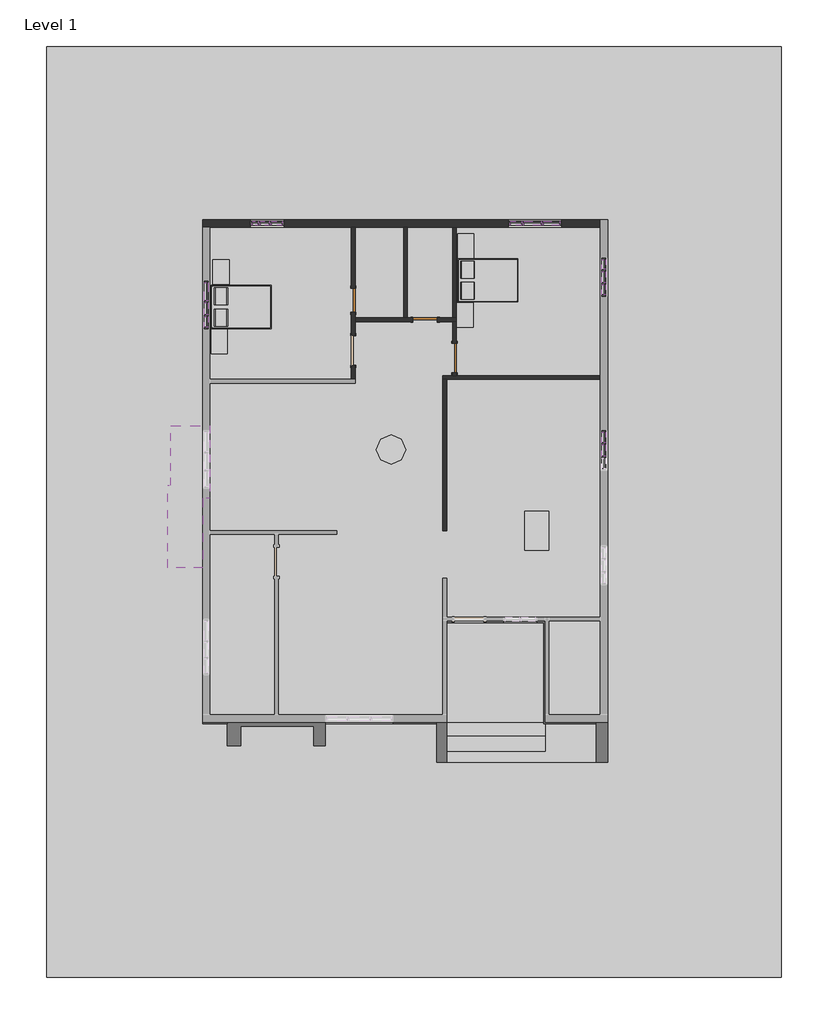
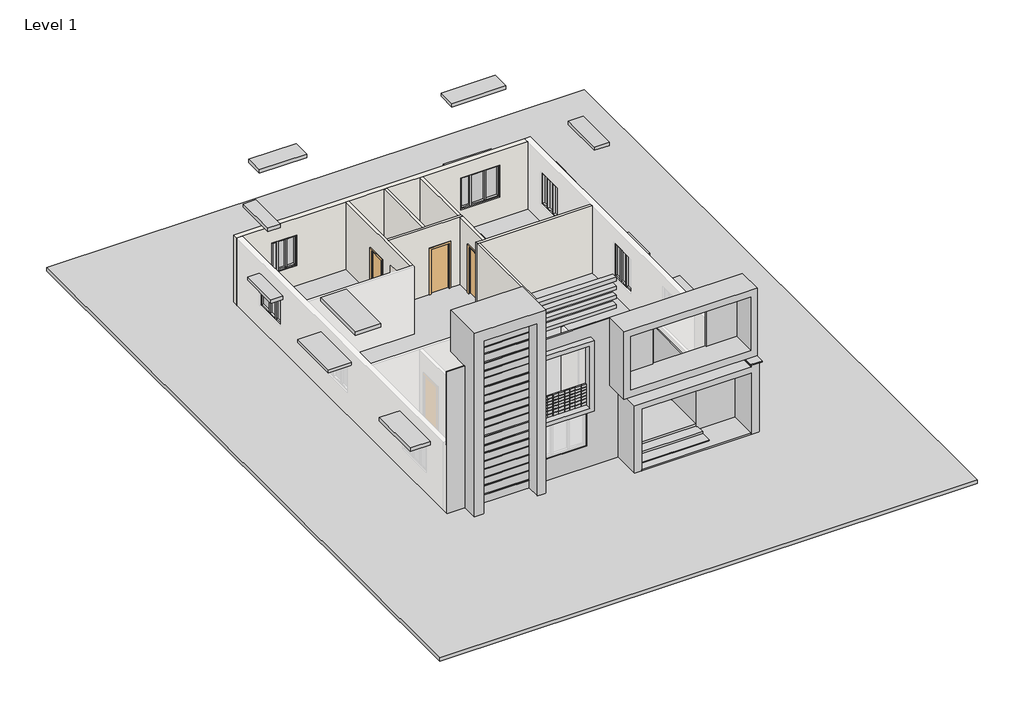
# One storey, part 2 of 2: 48 members, 14 plates, 8 furniture elements, 8 walls, 5 proxies, 3 doors.
"""IFC4 building model written with IfcOpenShell, lengths in millimetres."""

from ifc_helpers import new_model, si_unit, frame, origin, origin_with_axes, place, context, project, spatial, polyline, outline, extrude, faceted_brep, transform, mapped, element, save
from components import generic_models_1_generic_models_1_92a5afb8, generic_models_2_generic_models_2_c2d7a446, generic_models_3_generic_models_3_41235341, generic_models_4_generic_models_4_67bf9aa9, generic_models_6_generic_models_6_d9953a67, door_d8f5dbb5, door_f2b275c1, door_e5f9f3c4, furniture_b58f7881, furniture_fb07e05e, furniture_acc2807d, furniture_52f35bf4, member_ff1b7d8f, member_5ad95953, member_843225dc, member_ff9f2d30, member_49b269a4, member_6edf370a, member_39e99675, member_b57d713a, member_a980948f, member_0b7646a3, member_25243d18, member_408948b5, member_177aa30a, member_02b8d6b6, member_f68f0f88, member_d76d04ed, member_9890e23f, member_83c59054, member_6f432376, member_640288a7, member_b98e8178, system_panel_glazed_4b443884, system_panel_glazed_03b7eec7, system_panel_glazed_fe9977b0, system_panel_glazed_4bf0fdf0, system_panel_glazed_6a6571f5, system_panel_glazed_c4277b2e, system_panel_glazed_5760ca47, system_panel_glazed_ce423334, system_panel_glazed_199a1f6c, system_panel_glazed_e70e5af4, system_panel_glazed_65e788ca, system_panel_glazed_f9e68b79, system_panel_glazed_f010d5cf

model = new_model("IFC4")

# Units and contexts
model_context = context("Model", 3, world=origin())
ifc_project = project(units=[si_unit("LENGTHUNIT", "METRE", prefix="MILLI")], contexts=[model_context])

# Site, building, storey
site = spatial("IfcSite", under=ifc_project)
building = spatial("IfcBuilding", under=site)
storey = spatial("IfcBuildingStorey", under=building, Name="Level 1", Elevation=0.0)

# Proxies
placement = place(None, origin())
generic_models_1_generic_models_1_shape = generic_models_1_generic_models_1_92a5afb8(model_context)
element("IfcBuildingElementProxy", 1, Name="Generic Models 1 : Generic Models 1", ObjectType="Generic Models 1 : Generic Models 1", at=placement, inside=storey, context=model_context, shape_type="MappedRepresentation", body=[
    mapped(generic_models_1_generic_models_1_shape, transform((0.0, 0.0, 0.0), x_axis=(1.0, 0.0, 0.0), y_axis=(0.0, 1.0, 0.0), z_axis=(0.0, 0.0, 1.0))),
])
generic_models_2_generic_models_2_shape = generic_models_2_generic_models_2_c2d7a446(model_context)
element("IfcBuildingElementProxy", 2, Name="Generic Models 2 : Generic Models 2", ObjectType="Generic Models 2 : Generic Models 2", at=placement, inside=storey, context=model_context, shape_type="MappedRepresentation", body=[
    mapped(generic_models_2_generic_models_2_shape, transform((0.0, 0.0, 0.0), x_axis=(1.0, 0.0, 0.0), y_axis=(0.0, 1.0, 0.0), z_axis=(0.0, 0.0, 1.0))),
])
generic_models_3_generic_models_3_shape = generic_models_3_generic_models_3_41235341(model_context)
element("IfcBuildingElementProxy", 3, Name="Generic Models 3 : Generic Models 3", ObjectType="Generic Models 3 : Generic Models 3", at=placement, inside=storey, context=model_context, shape_type="MappedRepresentation", body=[
    mapped(generic_models_3_generic_models_3_shape, transform((0.0, 0.0, 0.0), x_axis=(1.0, 0.0, 0.0), y_axis=(0.0, 1.0, 0.0), z_axis=(0.0, 0.0, 1.0))),
])
generic_models_4_generic_models_4_shape = generic_models_4_generic_models_4_67bf9aa9(model_context)
element("IfcBuildingElementProxy", 4, Name="Generic Models 4 : Generic Models 4", ObjectType="Generic Models 4 : Generic Models 4", at=placement, inside=storey, context=model_context, shape_type="MappedRepresentation", body=[
    mapped(generic_models_4_generic_models_4_shape, transform((0.0, 0.0, 0.0), x_axis=(1.0, 0.0, 0.0), y_axis=(0.0, 1.0, 0.0), z_axis=(0.0, 0.0, 1.0))),
])
generic_models_6_generic_models_6_shape = generic_models_6_generic_models_6_d9953a67(model_context)
element("IfcBuildingElementProxy", 5, Name="Generic Models 6 : Generic Models 6", ObjectType="Generic Models 6 : Generic Models 6", at=placement, inside=storey, context=model_context, shape_type="MappedRepresentation", body=[
    mapped(generic_models_6_generic_models_6_shape, transform((0.0, 0.0, 0.0), x_axis=(1.0, 0.0, 0.0), y_axis=(0.0, 1.0, 0.0), z_axis=(0.0, 0.0, 1.0))),
])

# Doors
door_shape = door_d8f5dbb5(model_context)
element("IfcDoor", 6, ObjectType="Single-Flush : 30\" x 80\"", at=placement, inside=storey, context=model_context, shape_type="MappedRepresentation", body=[
    mapped(door_shape, transform((-18760.1886697, 977.9488046, 0.0), x_axis=(0.0, -1.0, 0.0), y_axis=(1.0, 0.0, 0.0), z_axis=(0.0, 0.0, 1.0))),
])
door_2_shape = door_f2b275c1(model_context)
element("IfcDoor", 7, ObjectType="Single-Flush : 30\" x 80\"", at=placement, inside=storey, context=model_context, shape_type="MappedRepresentation", body=[
    mapped(door_2_shape, transform((-16512.2886697, 368.3488046, 0.0), x_axis=(-1.0, 0.0, 0.0), y_axis=(0.0, -1.0, 0.0), z_axis=(0.0, 0.0, 1.0))),
])
door_3_shape = door_e5f9f3c4(model_context)
element("IfcDoor", 8, ObjectType="Single-Flush : 36\" x 84\"", at=placement, inside=storey, context=model_context, shape_type="MappedRepresentation", body=[
    mapped(door_3_shape, transform((-15597.8886697, -831.8011954, 0.0), x_axis=(0.0, -1.0, 0.0), y_axis=(1.0, 0.0, 0.0), z_axis=(0.0, 0.0, 1.0))),
])

# Furniture
furniture_shape = furniture_b58f7881(model_context)
element("IfcFurniture", 9, ObjectType="Bed-Box : Double 53\" x 74\"", at=placement, inside=storey, context=model_context, shape_type="MappedRepresentation", body=[
    mapped(furniture_shape, transform((-22493.4681779, 425.4988046, 0.0), x_axis=(0.0, 1.0, 0.0), y_axis=(-1.0, 0.0, 0.0), z_axis=(0.0, 0.0, 1.0))),
])
element("IfcFurniture", 10, ObjectType="Bed-Box : Double 53\" x 74\"", at=placement, inside=storey, context=model_context, shape_type="MappedRepresentation", body=[
    mapped(furniture_shape, transform((-14790.9181779, 1261.0963456, 0.0), x_axis=(0.0, 1.0, 0.0), y_axis=(-1.0, 0.0, 0.0), z_axis=(0.0, 0.0, 1.0))),
])
furniture_2_shape = furniture_fb07e05e(model_context)
element("IfcFurniture", 11, ObjectType="Cabinet File-Lateral 3 Drawer : 30\" x 20\" x 36\"", at=placement, inside=storey, context=model_context, shape_type="MappedRepresentation", body=[
    mapped(furniture_2_shape, transform((-23828.3570458, 2034.2713186, 0.0), x_axis=(0.0, 1.0, 0.0), y_axis=(-1.0, 0.0, 0.0), z_axis=(0.0, 0.0, 1.0))),
])
element("IfcFurniture", 12, ObjectType="Cabinet File-Lateral 3 Drawer : 30\" x 20\" x 36\"", at=placement, inside=storey, context=model_context, shape_type="MappedRepresentation", body=[
    mapped(furniture_2_shape, transform((-23879.1570458, -137.4286814, 0.0), x_axis=(0.0, 1.0, 0.0), y_axis=(-1.0, 0.0, 0.0), z_axis=(0.0, 0.0, 1.0))),
])
element("IfcFurniture", 13, ObjectType="Cabinet File-Lateral 3 Drawer : 30\" x 20\" x 36\"", at=placement, inside=storey, context=model_context, shape_type="MappedRepresentation", body=[
    mapped(furniture_2_shape, transform((-16176.6070458, 2847.0713186, 0.0), x_axis=(0.0, 1.0, 0.0), y_axis=(-1.0, 0.0, 0.0), z_axis=(0.0, 0.0, 1.0))),
])
element("IfcFurniture", 14, ObjectType="Cabinet File-Lateral 3 Drawer : 30\" x 20\" x 36\"", at=placement, inside=storey, context=model_context, shape_type="MappedRepresentation", body=[
    mapped(furniture_2_shape, transform((-16202.0070458, 700.7713186, 0.0), x_axis=(0.0, 1.0, 0.0), y_axis=(-1.0, 0.0, 0.0), z_axis=(0.0, 0.0, 1.0))),
])
furniture_3_shape = furniture_acc2807d(model_context)
element("IfcFurniture", 15, ObjectType="Table-Coffee Rectangular : 48\" x 30\"", at=placement, inside=storey, context=model_context, shape_type="MappedRepresentation", body=[
    mapped(furniture_3_shape, transform((-12656.5278379, -6836.2848256, 0.0), x_axis=(0.0, 1.0, 0.0), y_axis=(-1.0, 0.0, 0.0), z_axis=(0.0, 0.0, 1.0))),
])
furniture_4_shape = furniture_52f35bf4(model_context)
element("IfcFurniture", 16, ObjectType="Table-Dining Round w Chairs : 36\" Diameter", at=placement, inside=storey, context=model_context, shape_type="MappedRepresentation", body=[
    mapped(furniture_4_shape, transform((-17682.7706369, -3504.4225068, 0.0), x_axis=(1.0, 0.0, 0.0), y_axis=(0.0, 1.0, 0.0), z_axis=(0.0, 0.0, 1.0))),
])

# Members
member_shape = member_ff1b7d8f(model_context)
element("IfcMember", 17, ObjectType="Rectangular Mullion : 2.5\" x 5\" rectangular", at=placement, inside=storey, context=model_context, shape_type="MappedRepresentation", body=[
    mapped(member_shape, transform((-10930.6386697, 1530.3988046, 2267.0732017), x_axis=(0.0, 0.0, 1.0), y_axis=(-1.0, 0.0, 0.0), z_axis=(0.0, -1.0, 0.0))),
])
member_2_shape = member_5ad95953(model_context)
element("IfcMember", 18, ObjectType="Rectangular Mullion : 2.5\" x 5\" rectangular", at=placement, inside=storey, context=model_context, shape_type="MappedRepresentation", body=[
    mapped(member_2_shape, transform((-10930.6386697, 1936.7988046, 2267.0732017), x_axis=(0.0, 0.0, 1.0), y_axis=(-1.0, 0.0, 0.0), z_axis=(0.0, -1.0, 0.0))),
])
element("IfcMember", 19, ObjectType="Rectangular Mullion : 2.5\" x 5\" rectangular", at=placement, inside=storey, context=model_context, shape_type="MappedRepresentation", body=[
    mapped(member_2_shape, transform((-10930.6386697, 1155.7488046, 2267.0732017), x_axis=(0.0, 0.0, 1.0), y_axis=(-1.0, 0.0, 0.0), z_axis=(0.0, -1.0, 0.0))),
])
element("IfcMember", 20, ObjectType="Rectangular Mullion : 2.5\" x 5\" rectangular", at=placement, inside=storey, context=model_context, shape_type="MappedRepresentation", body=[
    mapped(member_2_shape, transform((-10930.6386697, 1466.8988046, 809.8934331), x_axis=(0.0, 0.0, -1.0), y_axis=(-1.0, 0.0, 0.0), z_axis=(0.0, 1.0, 0.0))),
])
element("IfcMember", 21, ObjectType="Rectangular Mullion : 2.5\" x 5\" rectangular", at=placement, inside=storey, context=model_context, shape_type="MappedRepresentation", body=[
    mapped(member_2_shape, transform((-10930.6386697, 2247.9488046, 809.8934331), x_axis=(0.0, 0.0, -1.0), y_axis=(-1.0, 0.0, 0.0), z_axis=(0.0, 1.0, 0.0))),
])
element("IfcMember", 22, ObjectType="Rectangular Mullion : 2.5\" x 5\" rectangular", at=placement, inside=storey, context=model_context, shape_type="MappedRepresentation", body=[
    mapped(member_shape, transform((-10930.6386697, 1873.2988046, 809.8934331), x_axis=(0.0, 0.0, -1.0), y_axis=(-1.0, 0.0, 0.0), z_axis=(0.0, 1.0, 0.0))),
])
member_3_shape = member_843225dc(model_context)
element("IfcMember", 23, ObjectType="Rectangular Mullion : 2.5\" x 5\" rectangular", at=placement, inside=storey, context=model_context, shape_type="MappedRepresentation", body=[
    mapped(member_3_shape, transform((-10930.6386697, -3536.9011954, 821.4712655), x_axis=(0.0, 0.0, -1.0), y_axis=(-1.0, 0.0, 0.0), z_axis=(0.0, 1.0, 0.0))),
])
element("IfcMember", 24, ObjectType="Rectangular Mullion : 2.5\" x 5\" rectangular", at=placement, inside=storey, context=model_context, shape_type="MappedRepresentation", body=[
    mapped(member_3_shape, transform((-13857.9886697, 3378.2488046, 969.97905), x_axis=(0.0, 0.0, -1.0), y_axis=(0.0, -1.0, 0.0), z_axis=(-1.0, 0.0, 0.0))),
])
member_4_shape = member_ff9f2d30(model_context)
element("IfcMember", 25, ObjectType="Rectangular Mullion : 2.5\" x 5\" rectangular", at=placement, inside=storey, context=model_context, shape_type="MappedRepresentation", body=[
    mapped(member_4_shape, transform((-10930.6386697, -3962.3511954, 821.4712655), x_axis=(0.0, 0.0, -1.0), y_axis=(-1.0, 0.0, 0.0), z_axis=(0.0, 1.0, 0.0))),
])
element("IfcMember", 26, ObjectType="Rectangular Mullion : 2.5\" x 5\" rectangular", at=placement, inside=storey, context=model_context, shape_type="MappedRepresentation", body=[
    mapped(member_4_shape, transform((-10930.6386697, -3143.2011954, 821.4712655), x_axis=(0.0, 0.0, -1.0), y_axis=(-1.0, 0.0, 0.0), z_axis=(0.0, 1.0, 0.0))),
])
member_5_shape = member_49b269a4(model_context)
element("IfcMember", 27, ObjectType="Rectangular Mullion : 2.5\" x 5\" rectangular", at=placement, inside=storey, context=model_context, shape_type="MappedRepresentation", body=[
    mapped(member_5_shape, transform((-10930.6386697, -3930.6011954, 821.4712655), x_axis=(0.0, -1.0, 0.0), y_axis=(-1.0, 0.0, 0.0), z_axis=(0.0, 0.0, -1.0))),
])
element("IfcMember", 28, ObjectType="Rectangular Mullion : 2.5\" x 5\" rectangular", at=placement, inside=storey, context=model_context, shape_type="MappedRepresentation", body=[
    mapped(member_5_shape, transform((-10930.6386697, -3505.1511954, 821.4712655), x_axis=(0.0, -1.0, 0.0), y_axis=(-1.0, 0.0, 0.0), z_axis=(0.0, 0.0, -1.0))),
])
element("IfcMember", 29, ObjectType="Rectangular Mullion : 2.5\" x 5\" rectangular", at=placement, inside=storey, context=model_context, shape_type="MappedRepresentation", body=[
    mapped(member_3_shape, transform((-10930.6386697, -3898.8511954, 2353.4996799), x_axis=(0.0, 0.0, 1.0), y_axis=(-1.0, 0.0, 0.0), z_axis=(0.0, -1.0, 0.0))),
])
element("IfcMember", 30, ObjectType="Rectangular Mullion : 2.5\" x 5\" rectangular", at=placement, inside=storey, context=model_context, shape_type="MappedRepresentation", body=[
    mapped(member_3_shape, transform((-13496.0386697, 3378.2488046, 2411.6935747), x_axis=(0.0, 0.0, 1.0), y_axis=(0.0, -1.0, 0.0), z_axis=(1.0, 0.0, 0.0))),
])
element("IfcMember", 31, ObjectType="Rectangular Mullion : 2.5\" x 5\" rectangular", at=placement, inside=storey, context=model_context, shape_type="MappedRepresentation", body=[
    mapped(member_4_shape, transform((-10930.6386697, -3473.4011954, 2353.4996799), x_axis=(0.0, 0.0, 1.0), y_axis=(-1.0, 0.0, 0.0), z_axis=(0.0, -1.0, 0.0))),
])
member_6_shape = member_6edf370a(model_context)
element("IfcMember", 32, ObjectType="Rectangular Mullion : 2.5\" x 5\" rectangular", at=placement, inside=storey, context=model_context, shape_type="MappedRepresentation", body=[
    mapped(member_6_shape, transform((-10930.6386697, -3079.7011954, 2353.4996799), x_axis=(0.0, 1.0, 0.0), y_axis=(-1.0, 0.0, 0.0), z_axis=(0.0, 0.0, 1.0))),
])
member_7_shape = member_39e99675(model_context)
element("IfcMember", 33, ObjectType="Rectangular Mullion : 2.5\" x 5\" rectangular", at=placement, inside=storey, context=model_context, shape_type="MappedRepresentation", body=[
    mapped(member_7_shape, transform((-10930.6386697, 1498.6488046, 809.8934331), x_axis=(0.0, -1.0, 0.0), y_axis=(-1.0, 0.0, 0.0), z_axis=(0.0, 0.0, -1.0))),
])
element("IfcMember", 34, ObjectType="Rectangular Mullion : 2.5\" x 5\" rectangular", at=placement, inside=storey, context=model_context, shape_type="MappedRepresentation", body=[
    mapped(member_7_shape, transform((-10930.6386697, 1905.0488046, 809.8934331), x_axis=(0.0, -1.0, 0.0), y_axis=(-1.0, 0.0, 0.0), z_axis=(0.0, 0.0, -1.0))),
])
member_8_shape = member_b57d713a(model_context)
element("IfcMember", 35, ObjectType="Rectangular Mullion : 2.5\" x 5\" rectangular", at=placement, inside=storey, context=model_context, shape_type="MappedRepresentation", body=[
    mapped(member_8_shape, transform((-10930.6386697, 1092.2488046, 809.8934331), x_axis=(0.0, -1.0, 0.0), y_axis=(-1.0, 0.0, 0.0), z_axis=(0.0, 0.0, -1.0))),
])
element("IfcMember", 36, ObjectType="Rectangular Mullion : 2.5\" x 5\" rectangular", at=placement, inside=storey, context=model_context, shape_type="MappedRepresentation", body=[
    mapped(member_8_shape, transform((-10930.6386697, 2311.4488046, 2267.0732017), x_axis=(0.0, 1.0, 0.0), y_axis=(-1.0, 0.0, 0.0), z_axis=(0.0, 0.0, 1.0))),
])
member_9_shape = member_a980948f(model_context)
element("IfcMember", 37, ObjectType="Rectangular Mullion : 2.5\" x 5\" rectangular", at=placement, inside=storey, context=model_context, shape_type="MappedRepresentation", body=[
    mapped(member_9_shape, transform((-12886.4386697, 3378.2488046, 2411.6935747), x_axis=(0.0, 0.0, 1.0), y_axis=(0.0, -1.0, 0.0), z_axis=(1.0, 0.0, 0.0))),
])
member_10_shape = member_0b7646a3(model_context)
element("IfcMember", 38, ObjectType="Rectangular Mullion : 2.5\" x 5\" rectangular", at=placement, inside=storey, context=model_context, shape_type="MappedRepresentation", body=[
    mapped(member_10_shape, transform((-12308.5886697, 3378.2488046, 2411.6935747), x_axis=(0.0, 0.0, 1.0), y_axis=(0.0, -1.0, 0.0), z_axis=(1.0, 0.0, 0.0))),
])
member_11_shape = member_25243d18(model_context)
element("IfcMember", 39, ObjectType="Rectangular Mullion : 2.5\" x 5\" rectangular", at=placement, inside=storey, context=model_context, shape_type="MappedRepresentation", body=[
    mapped(member_11_shape, transform((-12854.6886697, 3378.2488046, 969.97905), x_axis=(1.0, 0.0, 0.0), y_axis=(0.0, -1.0, 0.0), z_axis=(0.0, 0.0, -1.0))),
])
element("IfcMember", 40, ObjectType="Rectangular Mullion : 2.5\" x 5\" rectangular", at=placement, inside=storey, context=model_context, shape_type="MappedRepresentation", body=[
    mapped(member_11_shape, transform((-13464.2886697, 3378.2488046, 969.97905), x_axis=(1.0, 0.0, 0.0), y_axis=(0.0, -1.0, 0.0), z_axis=(0.0, 0.0, -1.0))),
])
element("IfcMember", 41, ObjectType="Rectangular Mullion : 2.5\" x 5\" rectangular", at=placement, inside=storey, context=model_context, shape_type="MappedRepresentation", body=[
    mapped(member_10_shape, transform((-12822.9386697, 3378.2488046, 969.97905), x_axis=(0.0, 0.0, -1.0), y_axis=(0.0, -1.0, 0.0), z_axis=(-1.0, 0.0, 0.0))),
])
element("IfcMember", 42, ObjectType="Rectangular Mullion : 2.5\" x 5\" rectangular", at=placement, inside=storey, context=model_context, shape_type="MappedRepresentation", body=[
    mapped(member_9_shape, transform((-13432.5386697, 3378.2488046, 969.97905), x_axis=(0.0, 0.0, -1.0), y_axis=(0.0, -1.0, 0.0), z_axis=(-1.0, 0.0, 0.0))),
])
member_12_shape = member_408948b5(model_context)
element("IfcMember", 43, ObjectType="Rectangular Mullion : 2.5\" x 5\" rectangular", at=placement, inside=storey, context=model_context, shape_type="MappedRepresentation", body=[
    mapped(member_12_shape, transform((-12245.0886697, 3378.2488046, 969.97905), x_axis=(1.0, 0.0, 0.0), y_axis=(0.0, -1.0, 0.0), z_axis=(0.0, 0.0, -1.0))),
])
element("IfcMember", 44, ObjectType="Rectangular Mullion : 2.5\" x 5\" rectangular", at=placement, inside=storey, context=model_context, shape_type="MappedRepresentation", body=[
    mapped(member_12_shape, transform((-13921.4886697, 3378.2488046, 2411.6935747), x_axis=(-1.0, 0.0, 0.0), y_axis=(0.0, -1.0, 0.0), z_axis=(0.0, 0.0, 1.0))),
])
member_13_shape = member_177aa30a(model_context)
element("IfcMember", 45, ObjectType="Rectangular Mullion : 2.5\" x 5\" rectangular", at=placement, inside=storey, context=model_context, shape_type="MappedRepresentation", body=[
    mapped(member_13_shape, transform((-21376.3886697, 3378.2488046, 2287.6988382), x_axis=(0.0, 0.0, 1.0), y_axis=(0.0, -1.0, 0.0), z_axis=(1.0, 0.0, 0.0))),
])
member_14_shape = member_02b8d6b6(model_context)
element("IfcMember", 46, ObjectType="Rectangular Mullion : 2.5\" x 5\" rectangular", at=placement, inside=storey, context=model_context, shape_type="MappedRepresentation", body=[
    mapped(member_14_shape, transform((-20976.3386697, 3378.2488046, 2287.6988382), x_axis=(0.0, 0.0, 1.0), y_axis=(0.0, -1.0, 0.0), z_axis=(1.0, 0.0, 0.0))),
])
element("IfcMember", 47, ObjectType="Rectangular Mullion : 2.5\" x 5\" rectangular", at=placement, inside=storey, context=model_context, shape_type="MappedRepresentation", body=[
    mapped(member_14_shape, transform((-23351.2386697, 127.0488046, 2332.8596388), x_axis=(0.0, 0.0, 1.0), y_axis=(-1.0, 0.0, 0.0), z_axis=(0.0, -1.0, 0.0))),
])
member_15_shape = member_f68f0f88(model_context)
element("IfcMember", 48, ObjectType="Rectangular Mullion : 2.5\" x 5\" rectangular", at=placement, inside=storey, context=model_context, shape_type="MappedRepresentation", body=[
    mapped(member_15_shape, transform((-21344.6386697, 3378.2488046, 911.0651886), x_axis=(1.0, 0.0, 0.0), y_axis=(0.0, -1.0, 0.0), z_axis=(0.0, 0.0, -1.0))),
])
element("IfcMember", 49, ObjectType="Rectangular Mullion : 2.5\" x 5\" rectangular", at=placement, inside=storey, context=model_context, shape_type="MappedRepresentation", body=[
    mapped(member_15_shape, transform((-21700.2386697, 3378.2488046, 911.0651886), x_axis=(1.0, 0.0, 0.0), y_axis=(0.0, -1.0, 0.0), z_axis=(0.0, 0.0, -1.0))),
])
element("IfcMember", 50, ObjectType="Rectangular Mullion : 2.5\" x 5\" rectangular", at=placement, inside=storey, context=model_context, shape_type="MappedRepresentation", body=[
    mapped(member_13_shape, transform((-21668.4886697, 3378.2488046, 911.0651886), x_axis=(0.0, 0.0, -1.0), y_axis=(0.0, -1.0, 0.0), z_axis=(-1.0, 0.0, 0.0))),
])
element("IfcMember", 51, ObjectType="Rectangular Mullion : 2.5\" x 5\" rectangular", at=placement, inside=storey, context=model_context, shape_type="MappedRepresentation", body=[
    mapped(member_14_shape, transform((-21312.8886697, 3378.2488046, 911.0651886), x_axis=(0.0, 0.0, -1.0), y_axis=(0.0, -1.0, 0.0), z_axis=(-1.0, 0.0, 0.0))),
])
element("IfcMember", 52, ObjectType="Rectangular Mullion : 2.5\" x 5\" rectangular", at=placement, inside=storey, context=model_context, shape_type="MappedRepresentation", body=[
    mapped(member_14_shape, transform((-23351.2386697, 463.5988046, 1017.4338808), x_axis=(0.0, 0.0, -1.0), y_axis=(-1.0, 0.0, 0.0), z_axis=(0.0, 1.0, 0.0))),
])
member_16_shape = member_d76d04ed(model_context)
element("IfcMember", 53, ObjectType="Rectangular Mullion : 2.5\" x 5\" rectangular", at=placement, inside=storey, context=model_context, shape_type="MappedRepresentation", body=[
    mapped(member_16_shape, transform((-20912.8386697, 3378.2488046, 911.0651886), x_axis=(1.0, 0.0, 0.0), y_axis=(0.0, -1.0, 0.0), z_axis=(0.0, 0.0, -1.0))),
])
member_17_shape = member_9890e23f(model_context)
element("IfcMember", 54, ObjectType="Rectangular Mullion : 2.5\" x 5\" rectangular", at=placement, inside=storey, context=model_context, shape_type="MappedRepresentation", body=[
    mapped(member_17_shape, transform((-21731.9886697, 3378.2488046, 2287.6988382), x_axis=(0.0, 0.0, 1.0), y_axis=(0.0, -1.0, 0.0), z_axis=(1.0, 0.0, 0.0))),
])
element("IfcMember", 55, ObjectType="Rectangular Mullion : 2.5\" x 5\" rectangular", at=placement, inside=storey, context=model_context, shape_type="MappedRepresentation", body=[
    mapped(member_17_shape, transform((-21916.1386697, 3378.2488046, 911.0651886), x_axis=(0.0, 0.0, -1.0), y_axis=(0.0, -1.0, 0.0), z_axis=(-1.0, 0.0, 0.0))),
])
element("IfcMember", 56, ObjectType="Rectangular Mullion : 2.5\" x 5\" rectangular", at=placement, inside=storey, context=model_context, shape_type="MappedRepresentation", body=[
    mapped(member_16_shape, transform((-21979.6386697, 3378.2488046, 2287.6988382), x_axis=(-1.0, 0.0, 0.0), y_axis=(0.0, -1.0, 0.0), z_axis=(0.0, 0.0, 1.0))),
])
member_18_shape = member_83c59054(model_context)
element("IfcMember", 57, ObjectType="Rectangular Mullion : 2.5\" x 5\" rectangular", at=placement, inside=storey, context=model_context, shape_type="MappedRepresentation", body=[
    mapped(member_18_shape, transform((-23351.2386697, 527.0988046, 2332.8596388), x_axis=(0.0, 0.0, 1.0), y_axis=(-1.0, 0.0, 0.0), z_axis=(0.0, -1.0, 0.0))),
])
member_19_shape = member_6f432376(model_context)
element("IfcMember", 58, ObjectType="Rectangular Mullion : 2.5\" x 5\" rectangular", at=placement, inside=storey, context=model_context, shape_type="MappedRepresentation", body=[
    mapped(member_19_shape, transform((-23351.2386697, 958.8988046, 2332.8596388), x_axis=(0.0, 0.0, 1.0), y_axis=(-1.0, 0.0, 0.0), z_axis=(0.0, -1.0, 0.0))),
])
member_20_shape = member_640288a7(model_context)
element("IfcMember", 59, ObjectType="Rectangular Mullion : 2.5\" x 5\" rectangular", at=placement, inside=storey, context=model_context, shape_type="MappedRepresentation", body=[
    mapped(member_20_shape, transform((-23351.2386697, 927.1488046, 1017.4338808), x_axis=(0.0, -1.0, 0.0), y_axis=(-1.0, 0.0, 0.0), z_axis=(0.0, 0.0, -1.0))),
])
element("IfcMember", 60, ObjectType="Rectangular Mullion : 2.5\" x 5\" rectangular", at=placement, inside=storey, context=model_context, shape_type="MappedRepresentation", body=[
    mapped(member_20_shape, transform((-23351.2386697, 495.3488046, 1017.4338808), x_axis=(0.0, -1.0, 0.0), y_axis=(-1.0, 0.0, 0.0), z_axis=(0.0, 0.0, -1.0))),
])
element("IfcMember", 61, ObjectType="Rectangular Mullion : 2.5\" x 5\" rectangular", at=placement, inside=storey, context=model_context, shape_type="MappedRepresentation", body=[
    mapped(member_18_shape, transform((-23351.2386697, 895.3988046, 1017.4338808), x_axis=(0.0, 0.0, -1.0), y_axis=(-1.0, 0.0, 0.0), z_axis=(0.0, 1.0, 0.0))),
])
element("IfcMember", 62, ObjectType="Rectangular Mullion : 2.5\" x 5\" rectangular", at=placement, inside=storey, context=model_context, shape_type="MappedRepresentation", body=[
    mapped(member_19_shape, transform((-23351.2386697, 1524.0488046, 1017.4338808), x_axis=(0.0, 0.0, -1.0), y_axis=(-1.0, 0.0, 0.0), z_axis=(0.0, 1.0, 0.0))),
])
member_21_shape = member_b98e8178(model_context)
element("IfcMember", 63, ObjectType="Rectangular Mullion : 2.5\" x 5\" rectangular", at=placement, inside=storey, context=model_context, shape_type="MappedRepresentation", body=[
    mapped(member_21_shape, transform((-23351.2386697, 63.5488046, 1017.4338808), x_axis=(0.0, -1.0, 0.0), y_axis=(-1.0, 0.0, 0.0), z_axis=(0.0, 0.0, -1.0))),
])
element("IfcMember", 64, ObjectType="Rectangular Mullion : 2.5\" x 5\" rectangular", at=placement, inside=storey, context=model_context, shape_type="MappedRepresentation", body=[
    mapped(member_21_shape, transform((-23351.2386697, 1587.5488046, 2332.8596388), x_axis=(0.0, 1.0, 0.0), y_axis=(-1.0, 0.0, 0.0), z_axis=(0.0, 0.0, 1.0))),
])

# Plates
system_panel_glazed_shape = system_panel_glazed_4b443884(model_context)
element("IfcPlate", 65, ObjectType="System Panel : Glazed", at=placement, inside=storey, context=model_context, shape_type="MappedRepresentation", body=[
    mapped(system_panel_glazed_shape, transform((-10930.6386697, -3308.3011954, 884.9712655), x_axis=(0.0, -1.0, 0.0), y_axis=(1.0, 0.0, 0.0), z_axis=(0.0, 0.0, 1.0))),
])
system_panel_glazed_2_shape = system_panel_glazed_03b7eec7(model_context)
element("IfcPlate", 66, ObjectType="System Panel : Glazed", at=placement, inside=storey, context=model_context, shape_type="MappedRepresentation", body=[
    mapped(system_panel_glazed_2_shape, transform((-10930.6386697, -3717.8761954, 884.9712655), x_axis=(0.0, -1.0, 0.0), y_axis=(1.0, 0.0, 0.0), z_axis=(0.0, 0.0, 1.0))),
])
system_panel_glazed_3_shape = system_panel_glazed_fe9977b0(model_context)
element("IfcPlate", 67, ObjectType="System Panel : Glazed", at=placement, inside=storey, context=model_context, shape_type="MappedRepresentation", body=[
    mapped(system_panel_glazed_3_shape, transform((-10930.6386697, 2092.3738046, 873.3934331), x_axis=(0.0, -1.0, 0.0), y_axis=(1.0, 0.0, 0.0), z_axis=(0.0, 0.0, 1.0))),
])
element("IfcPlate", 68, ObjectType="System Panel : Glazed", at=placement, inside=storey, context=model_context, shape_type="MappedRepresentation", body=[
    mapped(system_panel_glazed_3_shape, transform((-10930.6386697, 1311.3238046, 873.3934331), x_axis=(0.0, -1.0, 0.0), y_axis=(1.0, 0.0, 0.0), z_axis=(0.0, 0.0, 1.0))),
])
system_panel_glazed_4_shape = system_panel_glazed_4bf0fdf0(model_context)
element("IfcPlate", 69, ObjectType="System Panel : Glazed", at=placement, inside=storey, context=model_context, shape_type="MappedRepresentation", body=[
    mapped(system_panel_glazed_4_shape, transform((-10930.6386697, 1701.8488046, 873.3934331), x_axis=(0.0, -1.0, 0.0), y_axis=(1.0, 0.0, 0.0), z_axis=(0.0, 0.0, 1.0))),
])
system_panel_glazed_5_shape = system_panel_glazed_6a6571f5(model_context)
element("IfcPlate", 70, ObjectType="System Panel : Glazed", at=placement, inside=storey, context=model_context, shape_type="MappedRepresentation", body=[
    mapped(system_panel_glazed_5_shape, transform((-13159.4886697, 3378.2488046, 1033.47905), x_axis=(1.0, 0.0, 0.0), y_axis=(0.0, 1.0, 0.0), z_axis=(0.0, 0.0, 1.0))),
])
system_panel_glazed_6_shape = system_panel_glazed_c4277b2e(model_context)
element("IfcPlate", 71, ObjectType="System Panel : Glazed", at=placement, inside=storey, context=model_context, shape_type="MappedRepresentation", body=[
    mapped(system_panel_glazed_6_shape, transform((-12565.7636697, 3378.2488046, 1033.47905), x_axis=(1.0, 0.0, 0.0), y_axis=(0.0, 1.0, 0.0), z_axis=(0.0, 0.0, 1.0))),
])
system_panel_glazed_7_shape = system_panel_glazed_5760ca47(model_context)
element("IfcPlate", 72, ObjectType="System Panel : Glazed", at=placement, inside=storey, context=model_context, shape_type="MappedRepresentation", body=[
    mapped(system_panel_glazed_7_shape, transform((-13677.0136697, 3378.2488046, 1033.47905), x_axis=(1.0, 0.0, 0.0), y_axis=(0.0, 1.0, 0.0), z_axis=(0.0, 0.0, 1.0))),
])
system_panel_glazed_8_shape = system_panel_glazed_ce423334(model_context)
element("IfcPlate", 73, ObjectType="System Panel : Glazed", at=placement, inside=storey, context=model_context, shape_type="MappedRepresentation", body=[
    mapped(system_panel_glazed_8_shape, transform((-21144.6136697, 3378.2488046, 974.5651886), x_axis=(1.0, 0.0, 0.0), y_axis=(0.0, 1.0, 0.0), z_axis=(0.0, 0.0, 1.0))),
])
system_panel_glazed_9_shape = system_panel_glazed_199a1f6c(model_context)
element("IfcPlate", 74, ObjectType="System Panel : Glazed", at=placement, inside=storey, context=model_context, shape_type="MappedRepresentation", body=[
    mapped(system_panel_glazed_9_shape, transform((-21522.4386697, 3378.2488046, 974.5651886), x_axis=(1.0, 0.0, 0.0), y_axis=(0.0, 1.0, 0.0), z_axis=(0.0, 0.0, 1.0))),
])
system_panel_glazed_10_shape = system_panel_glazed_e70e5af4(model_context)
element("IfcPlate", 75, ObjectType="System Panel : Glazed", at=placement, inside=storey, context=model_context, shape_type="MappedRepresentation", body=[
    mapped(system_panel_glazed_10_shape, transform((-21824.0636697, 3378.2488046, 974.5651886), x_axis=(1.0, 0.0, 0.0), y_axis=(0.0, 1.0, 0.0), z_axis=(0.0, 0.0, 1.0))),
])
system_panel_glazed_11_shape = system_panel_glazed_65e788ca(model_context)
element("IfcPlate", 76, ObjectType="System Panel : Glazed", at=placement, inside=storey, context=model_context, shape_type="MappedRepresentation", body=[
    mapped(system_panel_glazed_11_shape, transform((-23351.2386697, 1241.4738046, 1080.9338808), x_axis=(0.0, -1.0, 0.0), y_axis=(1.0, 0.0, 0.0), z_axis=(0.0, 0.0, 1.0))),
])
system_panel_glazed_12_shape = system_panel_glazed_f9e68b79(model_context)
element("IfcPlate", 77, ObjectType="System Panel : Glazed", at=placement, inside=storey, context=model_context, shape_type="MappedRepresentation", body=[
    mapped(system_panel_glazed_12_shape, transform((-23351.2386697, 711.2488046, 1080.9338808), x_axis=(0.0, -1.0, 0.0), y_axis=(1.0, 0.0, 0.0), z_axis=(0.0, 0.0, 1.0))),
])
system_panel_glazed_13_shape = system_panel_glazed_f010d5cf(model_context)
element("IfcPlate", 78, ObjectType="System Panel : Glazed", at=placement, inside=storey, context=model_context, shape_type="MappedRepresentation", body=[
    mapped(system_panel_glazed_13_shape, transform((-23351.2386697, 295.3238046, 1080.9338808), x_axis=(0.0, -1.0, 0.0), y_axis=(1.0, 0.0, 0.0), z_axis=(0.0, 0.0, 1.0))),
])

# Walls
element("IfcWall", 79, ObjectType="4.5\"", at=placement, inside=storey, context=model_context, shape_type="Brep", body=[
    faceted_brep([(-18703.0386697, -136.4761954, 0.0), (-18703.0386697, 311.1988046, 0.0), (-18703.0386697, 425.4988046, 0.0), (-18703.0386697, 596.9488046, 0.0), (-18703.0386697, 596.9488046, 2032.0), (-18703.0386697, 1358.9488046, 2032.0), (-18703.0386697, 1358.9488046, 0.0), (-18703.0386697, 3263.9488046, 0.0), (-18703.0386697, 3263.9488046, 3048.0), (-18703.0386697, 425.4988046, 3048.0), (-18703.0386697, 311.1988046, 3048.0), (-18703.0386697, -1498.5511954, 3048.0), (-18703.0386697, -1498.5511954, 0.0), (-18703.0386697, -1050.8761954, 0.0), (-18703.0386697, -1050.8761954, 2133.6), (-18703.0386697, -136.4761954, 2133.6), (-18817.3386697, 596.9488046, 2032.0), (-18817.3386697, 596.9488046, 0.0), (-18817.3386697, -136.4761954, 0.0), (-18817.3386697, -136.4761954, 2133.6), (-18817.3386697, -1050.8761954, 2133.6), (-18817.3386697, -1050.8761954, 0.0), (-18817.3386697, -1498.5511954, 0.0), (-18817.3386697, -1498.5511954, 3048.0), (-18817.3386697, 3263.9488046, 3048.0), (-18817.3386697, 3263.9488046, 0.0), (-18817.3386697, 1358.9488046, 0.0), (-18817.3386697, 1358.9488046, 2032.0)], [[[0, 1, 2, 3, 4, 5, 6, 7, 8, 9, 10, 11, 12, 13, 14, 15]], [[16, 17, 18, 19, 20, 21, 22, 23, 24, 25, 26, 27]], [[13, 12, 22, 21]], [[26, 25, 7, 6]], [[18, 17, 3, 2, 1, 0]], [[11, 10, 9, 8, 24, 23]], [[12, 11, 23, 22]], [[8, 7, 25, 24]], [[19, 18, 0, 15]], [[20, 19, 15, 14]], [[21, 20, 14, 13]], [[4, 3, 17, 16]], [[5, 4, 16, 27]], [[6, 5, 27, 26]]]),
])
element("IfcWall", 80, ObjectType="4.5\"", at=placement, inside=storey, context=model_context, shape_type="Brep", body=[
    faceted_brep([(-18703.0386697, 311.1988046, 0.0), (-16893.2886697, 311.1988046, 0.0), (-16893.2886697, 311.1988046, 2032.0), (-16131.2886697, 311.1988046, 2032.0), (-16131.2886697, 311.1988046, 0.0), (-15655.0386697, 311.1988046, 0.0), (-15540.7386697, 311.1988046, 0.0), (-15540.7386697, 311.1988046, 3048.0), (-15655.0386697, 311.1988046, 3048.0), (-18703.0386697, 311.1988046, 3048.0), (-16893.2886697, 425.4988046, 2032.0), (-16893.2886697, 425.4988046, 0.0), (-17064.7386697, 425.4988046, 0.0), (-17179.0386697, 425.4988046, 0.0), (-18703.0386697, 425.4988046, 0.0), (-18703.0386697, 425.4988046, 3048.0), (-17179.0386697, 425.4988046, 3048.0), (-17064.7386697, 425.4988046, 3048.0), (-15655.0386697, 425.4988046, 3048.0), (-15540.7386697, 425.4988046, 3048.0), (-15540.7386697, 425.4988046, 0.0), (-15655.0386697, 425.4988046, 0.0), (-16131.2886697, 425.4988046, 0.0), (-16131.2886697, 425.4988046, 2032.0)], [[[0, 1, 2, 3, 4, 5, 6, 7, 8, 9]], [[10, 11, 12, 13, 14, 15, 16, 17, 18, 19, 20, 21, 22, 23]], [[22, 21, 20, 6, 5, 4]], [[14, 13, 12, 11, 1, 0]], [[9, 8, 7, 19, 18, 17, 16, 15]], [[0, 9, 15, 14]], [[7, 6, 20, 19]], [[2, 1, 11, 10]], [[3, 2, 10, 23]], [[4, 3, 23, 22]]]),
])
element("IfcWall", 81, ObjectType="4.5\"", at=placement, inside=storey, context=model_context, shape_type="SweptSolid", body=[
    extrude(outline(polyline([(-17064.7386697, 3263.9488046), (-17064.7386697, 425.4988046), (-17179.0386697, 425.4988046), (-17179.0386697, 3263.9488046), (-17064.7386697, 3263.9488046)])), origin_with_axes(), (0.0, 0.0, 1.0), 3048.0),
])
element("IfcWall", 82, ObjectType="4.5\"", at=placement, inside=storey, context=model_context, shape_type="SweptSolid", body=[
    extrude(outline(polyline([(-15540.7386697, 3263.9488046), (-15540.7386697, 425.4988046), (-15655.0386697, 425.4988046), (-15655.0386697, 3263.9488046), (-15540.7386697, 3263.9488046)])), origin_with_axes(), (0.0, 0.0, 1.0), 3048.0),
])
element("IfcWall", 83, ObjectType="4.5\"", at=placement, inside=storey, context=model_context, shape_type="Brep", body=[
    faceted_brep([(-11044.9386697, -1384.2511954, 0.0), (-15540.7386697, -1384.2511954, 0.0), (-15655.0386697, -1384.2511954, 0.0), (-15959.8386697, -1384.2511954, 0.0), (-15959.8386697, -1384.2511954, 3048.0), (-15655.0386697, -1384.2511954, 3048.0), (-15540.7386697, -1384.2511954, 3048.0), (-11044.9386697, -1384.2511954, 3048.0), (-11044.9386697, -1498.5511954, 0.0), (-11044.9386697, -1498.5511954, 3048.0), (-15845.5386697, -1498.5511954, 3048.0), (-15959.8386697, -1498.5511954, 3048.0), (-15959.8386697, -1498.5511954, 0.0), (-15845.5386697, -1498.5511954, 0.0)], [[[0, 1, 2, 3, 4, 5, 6, 7]], [[8, 9, 10, 11, 12, 13]], [[3, 2, 1, 0, 8, 13, 12]], [[7, 6, 5, 4, 11, 10, 9]], [[0, 7, 9, 8]], [[4, 3, 12, 11]]]),
])
element("IfcWall", 84, ObjectType="4.5\"", at=placement, inside=storey, context=model_context, shape_type="SweptSolid", body=[
    extrude(outline(polyline([(-15959.8386697, -6222.9511954), (-15959.8386697, -1498.5511954), (-15845.5386697, -1498.5511954), (-15845.5386697, -6222.9511954), (-15959.8386697, -6222.9511954)])), origin_with_axes(), (0.0, 0.0, 1.0), 3048.0),
])
element("IfcWall", 85, ObjectType="4.5\"", at=placement, inside=storey, context=model_context, shape_type="SweptSolid", body=[
    extrude(outline(polyline([(-1289.0011954, 2133.6), (-1289.0011954, 0.0), (-1384.2511954, 0.0), (-1384.2511954, 3048.0), (311.1988046, 3048.0), (311.1988046, 0.0), (-374.6011954, 0.0), (-374.6011954, 2133.6), (-1289.0011954, 2133.6)])), frame((-15655.0386697, 0.0, 0.0), z_axis=(1.0, 0.0, 0.0), x_axis=(0.0, 1.0, 0.0)), (0.0, 0.0, 1.0), 114.3),
])
element("IfcWall", 86, ObjectType="9\"", at=placement, inside=storey, context=model_context, shape_type="Brep", body=[
    faceted_brep([(-11044.9386697, 3492.5488046, 0.0), (-23465.5386697, 3492.5488046, 0.0), (-23465.5386697, 3492.5488046, 3048.0), (-11044.9386697, 3492.5488046, 3048.0), (-21979.6386697, 3492.5488046, 2287.6988382), (-21979.6386697, 3492.5488046, 911.0651886), (-20912.8386697, 3492.5488046, 911.0651886), (-20912.8386697, 3492.5488046, 2287.6988382), (-13921.4886697, 3492.5488046, 2411.6935747), (-13921.4886697, 3492.5488046, 969.97905), (-12245.0886697, 3492.5488046, 969.97905), (-12245.0886697, 3492.5488046, 2411.6935747), (-23465.5386697, 3263.9488046, 0.0), (-23236.9386697, 3263.9488046, 0.0), (-18817.3386697, 3263.9488046, 0.0), (-18703.0386697, 3263.9488046, 0.0), (-17179.0386697, 3263.9488046, 0.0), (-17064.7386697, 3263.9488046, 0.0), (-15655.0386697, 3263.9488046, 0.0), (-15540.7386697, 3263.9488046, 0.0), (-11044.9386697, 3263.9488046, 0.0), (-11044.9386697, 3263.9488046, 3048.0), (-15540.7386697, 3263.9488046, 3048.0), (-15655.0386697, 3263.9488046, 3048.0), (-17064.7386697, 3263.9488046, 3048.0), (-17179.0386697, 3263.9488046, 3048.0), (-18703.0386697, 3263.9488046, 3048.0), (-18817.3386697, 3263.9488046, 3048.0), (-23236.9386697, 3263.9488046, 3048.0), (-23465.5386697, 3263.9488046, 3048.0), (-21979.6386697, 3263.9488046, 911.0651886), (-21979.6386697, 3263.9488046, 2287.6988382), (-20912.8386697, 3263.9488046, 2287.6988382), (-20912.8386697, 3263.9488046, 911.0651886), (-13921.4886697, 3263.9488046, 969.97905), (-13921.4886697, 3263.9488046, 2411.6935747), (-12245.0886697, 3263.9488046, 2411.6935747), (-12245.0886697, 3263.9488046, 969.97905)], [[[0, 1, 2, 3], [4, 5, 6, 7], [8, 9, 10, 11]], [[12, 13, 14, 15, 16, 17, 18, 19, 20, 21, 22, 23, 24, 25, 26, 27, 28, 29], [30, 31, 32, 33], [34, 35, 36, 37]], [[1, 0, 20, 19, 18, 17, 16, 15, 14, 13, 12]], [[3, 2, 29, 28, 27, 26, 25, 24, 23, 22, 21]], [[0, 3, 21, 20]], [[2, 1, 12, 29]], [[4, 31, 30, 5]], [[31, 4, 7, 32]], [[32, 7, 6, 33]], [[5, 30, 33, 6]], [[34, 9, 8, 35]], [[35, 8, 11, 36]], [[36, 11, 10, 37]], [[9, 34, 37, 10]]]),
])

save(model, "model.ifc")

# Revit data of these elements
# Type "Single-Flush : 30\" x 80\""
#   Type Mark = "5"
#   Construction Type Id = "MDOOR"
#   Assembly Code = "C1020"
#   Analytic Construction = "Metal"
#   Thickness = 0' - 2"
#   Heat Transfer Coefficient (U) = 0.651978 BTU/(h·ft²·°F)
#   Height = 6' - 8"
#   Trim Projection Ext = 0' - 1"
#   Trim Projection Int = 0' - 1"
#   Trim Width = 0' - 3"
#   Width = 2' - 6"
#   Define Thermal Properties by = 1
#   Define Thermal Properties by = 1
#   Door Material = Door - Panel
#   Frame Material = Door - Frame
#   Visual Light Transmittance = 0
#   Solar Heat Gain Coefficient = 0
#   Function = (empty or 0)
#   Wall Closure = (empty or 0)
# Type "Single-Flush : 36\" x 84\""
#   Type Mark = "1"
#   Construction Type Id = "MDOOR"
#   Assembly Code = "C1020"
#   Analytic Construction = "Metal"
#   Thickness = 0' - 2"
#   Heat Transfer Coefficient (U) = 0.651978 BTU/(h·ft²·°F)
#   Height = 7' - 0"
#   Trim Projection Ext = 0' - 1"
#   Trim Projection Int = 0' - 1"
#   Trim Width = 0' - 3"
#   Width = 3' - 0"
#   Define Thermal Properties by = 1
#   Define Thermal Properties by = 1
#   Door Material = Door - Panel
#   Frame Material = Door - Frame
#   Visual Light Transmittance = 0
#   Solar Heat Gain Coefficient = 0
#   Function = (empty or 0)
#   Wall Closure = (empty or 0)
# Type "Bed-Box : Double 53\" x 74\""
#   Assembly Code = "E2020200"
#   Length = 6' - 2"
#   Width = 4' - 5"
#   Frame Material = Birch
#   Mattress Material = Linen, White
#   Default Elevation = 0
# Type "Cabinet File-Lateral 3 Drawer : 30\" x 20\" x 36\""
#   Assembly Code = "E2020200"
#   Depth = 1' - 8"
#   Height = 3' - 0"
#   Width = 2' - 6"
#   Material = Metal - Steel
#   Default Elevation = 0
# Type "Table-Coffee Rectangular : 48\" x 30\""
#   Assembly Code = "E2020200"
#   Height = 1' - 1"
#   Length = 4' - 0"
#   Width = 2' - 6"
#   Base Material = Metal - Chrome
#   Table Top Material = Glass - Clear, Grey
#   Default Elevation = 0
# Type "Table-Dining Round w Chairs : 36\" Diameter"
#   Assembly Code = "E2020200"
#   Radius = 1' - 6"
#   Diameter = 3' - 0"
#   Height = 2' - 6"
#   Chairs = 4
#   Base Material = Pine
#   Top Material = Laminate, Linen, Matte
#   Default Elevation = 0
# Type "Rectangular Mullion : 2.5\" x 5\" rectangular"
#   built-in parameter 1007304 = 0.416667 (stored number, unit not read)
#   built-in parameter 1007301 = 0.104167 (stored number, unit not read)
#   built-in parameter 1007300 = 0.104167 (stored number, unit not read)
# Type "System Panel : Glazed"
#   Construction Type Id = "GSP4R"
#   Analytic Construction = "1/8 in Pilkington single glazing"
#   Visual Light Transmittance = 0.9
#   Solar Heat Gain Coefficient = 0.86
#   Heat Transfer Coefficient (U) = 1.18115 BTU/(h·ft²·°F)
#   Define Thermal Properties by = 1
# Type "4.5\""
#   Assembly Code = "B2010"
#   Layers, outside or top first: 0' - 4 1/2" no material (function 1)
# Type "9\""
#   Assembly Code = "B2010"
#   Layers, outside or top first: 0' - 9" no material (function 1)
# Element 1 (IfcBuildingElementProxy, "Generic Models 1 : Generic Models 1")
#   Phase Created = New Construction
# Element 2 (IfcBuildingElementProxy, "Generic Models 2 : Generic Models 2")
#   Phase Created = New Construction
# Element 3 (IfcBuildingElementProxy, "Generic Models 3 : Generic Models 3")
#   Phase Created = New Construction
# Element 4 (IfcBuildingElementProxy, "Generic Models 4 : Generic Models 4")
#   Phase Created = New Construction
# Element 5 (IfcBuildingElementProxy, "Generic Models 6 : Generic Models 6")
#   Phase Created = New Construction
# Elements 6, 7 (IfcDoor, "Single-Flush : 30\" x 80\"")
#   Phase Created = New Construction
#   Materials on its faces: "Door - Frame", "Door - Panel"
# Element 8 (IfcDoor, "Single-Flush : 36\" x 84\"")
#   Phase Created = New Construction
#   Materials on its faces: "Door - Frame", "Door - Panel"
# Elements 9, 10 (IfcFurniture, "Bed-Box : Double 53\" x 74\"")
#   Phase Created = New Construction
#   Materials on its faces: "Birch", "Linen, White"
# Elements 11, 12, 13, 14 (IfcFurniture, "Cabinet File-Lateral 3 Drawer : 30\" x 20\" x 36\"")
#   Phase Created = New Construction
#   Materials on its faces: "Metal - Steel"
# Element 15 (IfcFurniture, "Table-Coffee Rectangular : 48\" x 30\"")
#   Phase Created = New Construction
#   Materials on its faces: "Metal - Chrome", "Glass - Clear, Grey"
# Element 16 (IfcFurniture, "Table-Dining Round w Chairs : 36\" Diameter")
#   Phase Created = New Construction
#   Materials on its faces: "Pine", "Laminate, Linen, Matte"
# Elements 17, 18, 19, 20, 21, 22, 23, 24, 25, 26, 27, 28, 29, 30, 31, 32, 33, 34, 35, 36, 37, 38, 39, 40, 41, 42, 43, 44, 45, 46, 47, 48, 49, 50, 51, 52, 53, 54, 55, 56, 57, 58, 59, 60, 61, 62, 63, 64 (IfcMember, "Rectangular Mullion : 2.5\" x 5\" rectangular")
#   Phase Created = New Construction
#   Materials on its faces: "Aluminum"
# Elements 65, 66, 67, 68, 69, 70, 71, 72, 73, 74, 75, 76, 77, 78 (IfcPlate, "System Panel : Glazed")
#   Phase Created = New Construction
#   Materials on its faces: "Glass"
# Elements 79, 80, 81, 82, 83, 84, 85 (IfcWall, "4.5\"")
#   Top Offset = 0' - 0"
#   Base Offset = 0' - 0"
#   Unconnected Height = 10' - 0"
#   wall height = 10' - 0"
#   Phase Created = New Construction
#   Base Constraint = Level 1
#   Materials on its faces: "Default Wall"
# Element 86 (IfcWall, "9\"")
#   Top Offset = 0' - 0"
#   Base Offset = 0' - 0"
#   Unconnected Height = 10' - 0"
#   wall height = 10' - 0"
#   Phase Created = New Construction
#   Base Constraint = Level 1
#   Materials on its faces: "Default Wall"
# Materials
#   "Door - Panel": class "Wood", colour RGB 210 159 95, transparency 0, Cost = 0
#   "Door - Frame": colour RGB 118 70 51, transparency 0, Cost = 0
#   "Birch": class "Wood", colour RGB 224 178 126, transparency 0, Description = "Betula Alleghaniensis", Cost = 0
#   "Linen, White": class "Textile", colour RGB 247 247 239, transparency 0, Description = "Linen, white", Cost = 0
#   "Metal - Steel": colour RGB 209 209 209, transparency 0
#   "Metal - Chrome": colour RGB 57 57 57, transparency 0
#   "Glass - Clear, Grey": colour RGB 252 255 255, transparency 0.64
#   "Pine": class "Wood", colour RGB 223 192 134, transparency 0, Description = "Pinus Echinata", Cost = 0
#   "Laminate, Linen, Matte": class "Plastic", colour RGB 249 239 230, transparency 0, Description = "Plastic Laminate - Linen, Matte", Cost = 0
#   "Aluminum": class "Metal", colour RGB 247 247 247, transparency 0, Description = "Aluminum 6061", Cost = 0
#   "Glass": class "Glass", colour RGB 0 128 192, transparency 0.75, Description = "Soda Lime Glass", Cost = 0
#   "Default Wall": colour RGB 128 128 128, transparency 0, Cost = 0
